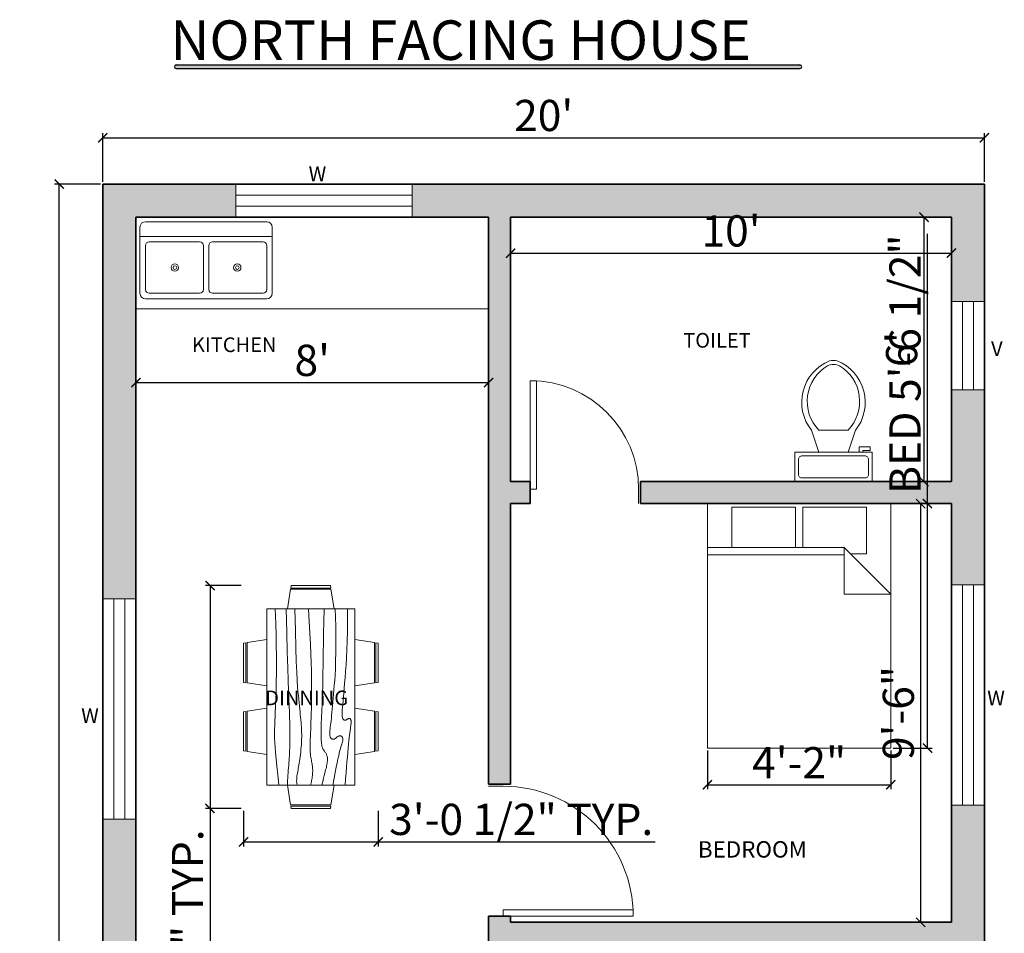
# Model space of a CAD drawing. Units: inches. Extents: x 3799 to 20199, y 1682 to 8087.
# Tile 29 of 30: x 17373 to 17641, y 7519 to 7768. Entities that reach past the tile are written whole.
import ezdxf

# ---------------------------------------------------------------- set-up
doc = ezdxf.new("R2010")
doc.units = ezdxf.units.IN
for name, color, linetype, lineweight in [('A-ANNO-DIMS', 2, 'Continuous', 18), ('A-ANNO-SYMB', 3, 'Continuous', 18), ('A-ANNO-TITL', 7, 'Continuous', 25), ('A-AREA-IDEN', 7, 'Continuous', 18), ('A-DOOR', 3, 'Continuous', 18), ('A-FLOR-CASE', 32, 'Continuous', 18), ('A-FLOR-FIXT', 9, 'Continuous', 18), ('A-FURN', 8, 'Continuous', 18), ('A-GLAZ', 152, 'Continuous', 18), ('A-WALL', 7, 'Continuous', 35), ('A-WALL-PATT', 252, 'Continuous', 13)]:
    doc.layers.add(name, color=color, linetype=linetype, lineweight=lineweight)
doc.styles.get("Standard").update_dxf_attribs({"font": 'arial.ttf'})
doc.dimstyles.new('ISO-25', dxfattribs={"dimtxt": 8.5, "dimasz": 2.5, "dimexe": 1.25, "dimexo": 0.625, "dimtad": 1, "dimdec": 0, "dimlunit": 3, "dimtxsty": 'Standard', "dimblk": 'ARCHTICK', "dimcen": 2.5, "dimadec": 0, "dimazin": 0, "dimtfac": 1, "dimtdec": 0, "dimtmove": 0, "dimatfit": 3, "dimfxl": 1, "dimarcsym": 0})

# ---------------------------------------------------------------- blocks, each defined once
blk = doc.blocks.new('*U47')
for p, q in [((0, 0), (0, -100)), ((750, 0), (750, -100))]:
    blk.add_line(p, q)
blk.add_lwpolyline([(0, 0), (0, 750), (43.75, 750), (43.75, 0)], close=True)
blk.add_arc((0, 0), 750, 0, 90)
blk = doc.blocks.new('*U124')
for p, q in [((0, 0), (0, -100)), ((-900, 0), (-900, -100))]:
    blk.add_line(p, q)
blk.add_lwpolyline([(0, 0), (0, 900), (-43.75, 900), (-43.75, 0)], close=True)
blk.add_arc((0, 0), 900, 90, 180)
blk = doc.blocks.new('Sink-double - 36 in top')
for p, q in [((-18, -4), (18, -4)), ((-0.75, -18.5), (-0.75, -6.5)), ((0.75, -6.5), (0.75, -18.5))]:
    blk.add_line(p, q)
for points in [[(-16.5, 0), (16.5, 0)], [(-18, -19.5), (-18, -1.5)], [(18, -1.5), (18, -19.5)], [(-16.5, -18.5), (-16.5, -6.5)], [(-15.5, -5.5), (-1.75, -5.5)], [(1.75, -5.5), (15.5, -5.5)], [(16.5, -6.5), (16.5, -18.5)], [(16.5, -21), (-16.5, -21)], [(-1.75, -19.5), (-15.5, -19.5)], [(15.5, -19.5), (1.75, -19.5)]]:
    blk.add_lwpolyline(points)
for centre, radius in [((-8.5, -12.5), 1), ((-8.5, -12.5), 0.5), ((8.5, -12.5), 1), ((8.5, -12.5), 0.5)]:
    blk.add_circle(centre, radius)
for centre, radius, start, end in [((-16.5, -1.5), 1.5, 90, 180), ((16.5, -1.5), 1.5, 0, 90), ((-15.5, -6.5), 1, 90, 180), ((-1.75, -6.5), 1, 0, 90), ((1.75, -6.5), 1, 90, 180), ((15.5, -6.5), 1, 0, 90), ((-15.5, -18.5), 1, 180, 270), ((-1.75, -18.5), 1, 270, 0), ((1.75, -18.5), 1, 180, 270), ((15.5, -18.5), 1, 270, 0), ((-16.5, -19.5), 1.5, 180, 270), ((16.5, -19.5), 1.5, 270, 0)]:
    blk.add_arc(centre, radius, start, end)
blk = doc.blocks.new('Toilet - top')
for p, q in [((9.5, -6), (9.5, -2)), ((-8, -8.5), (-8, -8)), ((-7, -8), (-7, -9.5)), ((-4, -8), (-6, -14)), ((4, -8), (6, -14)), ((-10, -8.5), (-8, -8.5)), ((-10, -9.5), (-10, -8.5)), ((-7, -9.5), (-10, -9.5)), ((4, -14), (-4, -14))]:
    blk.add_line(p, q)
blk.add_lwpolyline([(10.5, -8), (10.5, 0), (-10.5, 0), (-10.5, -8)], close=True)
for points in [[(-9.5, -2), (-9.5, -6)], [(8.5, -1), (-8.5, -1)], [(-8.5, -7), (8.5, -7)]]:
    blk.add_lwpolyline(points)
for centre, radius, start, end in [((-8.62, -1.88), 0.884, 81.8699, 188.1301), ((8.62, -1.88), 0.884, 351.8699, 98.1301), ((-8.62, -6.12), 0.884, 171.8699, 278.1301), ((8.62, -6.12), 0.884, 261.8699, 8.1301), ((3.52, -21.58), 12.17, 141.4691, 247.9714), ((4.2, -21.82), 11.33, 136.3677, 238.9468), ((-3.52, -21.58), 12.17, 292.0284, 38.5307), ((-4.2, -21.82), 11.33, 301.053, 43.6321), ((0, -27.88), 4, 245.7318, 294.2682), ((0, -29), 4, 254.8605, 285.1395)]:
    blk.add_arc(centre, radius, start, end)
blk = doc.blocks.new('Dining Set - 36 x 72 in.')
for p, q in [((-22.2343, 26.00059), (-23.4847, 17.99762)), ((-22.2304, 26), (-5.7608, 26)), ((-22, 27.5), (-22.1562, 26.50042)), ((-5.8416, 26.5), (-22.1534, 26.5)), ((-22, 27.5), (-6, 27.5)), ((-5.8437, 26.49966), (-6, 27.5)), ((-4.5152, 17.99762), (-5.7655, 25.99926)), ((5.7657, 26.00059), (4.5153, 17.99762)), ((5.7696, 26), (22.2392, 26)), ((6, 27.5), (5.8438, 26.50042)), ((22.1584, 26.5), (5.8466, 26.5)), ((6, 27.5), (22, 27.5)), ((22.1563, 26.49966), (22, 27.5)), ((23.4848, 17.99762), (22.2345, 25.99926)), ((36, 18), (-36, 18)), ((-36, 18), (-36, -18)), ((36, -18), (36, 18)), ((-45.5, 8), (-44.5004, 8.15617)), ((-44.5, -8.15843), (-44.5, 8.15338)), ((-44.0006, 8.23428), (-35.9976, 9.48474)), ((-44, 8.23041), (-44, -8.23915)), ((44.0006, 8.23428), (35.9976, 9.48474)), ((44, 8.23041), (44, -8.23915)), ((44.5, -8.15843), (44.5, 8.15338)), ((45.5, 8), (44.5005, 8.15617)), ((-45.5, 8), (-45.5, -8)), ((45.5, 8), (45.5, -8)), ((-44.4997, -8.15631), (-45.5, -8)), ((44.4997, -8.15631), (45.5, -8)), ((-35.9976, -9.48476), (-43.9993, -8.2345)), ((35.9976, -9.48476), (43.9993, -8.2345)), ((-36, -18), (36, -18)), ((-22.2343, -26.0006), (-23.4847, -17.99762)), ((-4.5152, -17.99762), (-5.7655, -25.99928)), ((5.7657, -26.0006), (4.5153, -17.99762)), ((23.4848, -17.99762), (22.2345, -25.99928)), ((-22.2304, -26), (-5.7608, -26)), ((-22, -27.5), (-22.1562, -26.50044)), ((-5.8416, -26.5), (-22.1534, -26.5)), ((-22, -27.5), (-6, -27.5)), ((-5.8437, -26.49967), (-6, -27.5)), ((5.7696, -26), (22.2392, -26)), ((6, -27.5), (5.8438, -26.50044)), ((22.1584, -26.5), (5.8466, -26.5)), ((6, -27.5), (22, -27.5)), ((22.1563, -26.49967), (22, -27.5))]:
    blk.add_line(p, q)
for points in [[(-36, 15), (-31.1772, 14.97754), (-26.8079, 14.91406), (-22.8538, 14.81543), (-19.276, 14.6875), (-16.0362, 14.53613), (-13.0957, 14.36718), (-10.4159, 14.18652), (-7.9583, 14), (-5.6904, 13.81315), (-3.6035, 13.63021), (-1.6954, 13.45508), (0.0365, 13.29166), (1.5945, 13.14388), (2.9811, 13.01562), (4.1988, 12.9108), (5.25, 12.83333), (6.1393, 12.78613), (6.8802, 12.76823), (7.4883, 12.77767), (7.9792, 12.8125), (8.3685, 12.87077), (8.6719, 12.95052), (8.9049, 13.0498), (9.0833, 13.16666), (9.2205, 13.29899), (9.3216, 13.44401), (9.3895, 13.59879), (9.4271, 13.76041), (9.4373, 13.92594), (9.4232, 14.09245), (9.3875, 14.257), (9.3333, 14.41666), (9.2638, 14.56917), (9.1836, 14.71484), (9.0975, 14.85465), (9.0104, 14.98958), (8.9272, 15.1206), (8.8529, 15.2487), (8.7922, 15.37483), (8.75, 15.5), (8.7305, 15.62467), (8.7344, 15.74739), (8.7617, 15.86621), (8.8125, 15.97916), (8.8867, 16.08431), (8.9844, 16.17968), (9.1055, 16.26334), (9.25, 16.33333), (9.4189, 16.38802), (9.6172, 16.42708), (9.8506, 16.45052), (10.125, 16.45833), (10.4463, 16.45052), (10.8203, 16.42708), (11.2529, 16.38802), (11.75, 16.33333), (12.3184, 16.26318), (12.9694, 16.17838), (13.7151, 16.07991), (14.5677, 15.96875), (15.5395, 15.84586), (16.6426, 15.71224), (17.8893, 15.56884), (19.2917, 15.41666), (20.859, 15.25667), (22.5879, 15.08984), (24.4721, 14.91715), (26.5052, 14.73958), (28.6809, 14.5581), (30.9929, 14.3737), (33.4347, 14.18733), (36, 14)], [(-36, 10), (-28.9766, 10.14274), (-23.1725, 10.20442), (-18.4241, 10.19775), (-14.5677, 10.13541), (-11.4399, 10.03011), (-8.877, 9.89453), (-6.7154, 9.74137), (-4.7917, 9.58333), (-2.9698, 9.43082), (-1.2246, 9.28515), (0.4415, 9.14534), (2.026, 9.01041), (3.5266, 8.87939), (4.9408, 8.7513), (6.266, 8.62516), (7.5, 8.5), (8.6411, 8.37549), (9.6914, 8.2539), (10.6538, 8.13818), (11.5312, 8.03125), (12.3267, 7.93603), (13.043, 7.85547), (13.6831, 7.79248), (14.25, 7.75), (14.7471, 7.7303), (15.1797, 7.73307), (15.5537, 7.75732), (15.875, 7.80208), (16.1494, 7.86637), (16.3828, 7.94922), (16.5811, 8.04964), (16.75, 8.16666), (16.8944, 8.29915), (17.0143, 8.44531), (17.1089, 8.60319), (17.1771, 8.77083), (17.218, 8.94629), (17.2305, 9.1276), (17.2137, 9.31282), (17.1667, 9.5), (17.0895, 9.6875), (16.987, 9.875), (16.8649, 10.0625), (16.7292, 10.25), (16.5856, 10.4375), (16.4401, 10.625), (16.2985, 10.8125), (16.1667, 11), (16.05, 11.18733), (15.9518, 11.3737), (15.8752, 11.5581), (15.8229, 11.73958), (15.798, 11.91715), (15.8034, 12.08984), (15.842, 12.25667), (15.9167, 12.41666), (16.0295, 12.56836), (16.1784, 12.70833), (16.3605, 12.83268), (16.5729, 12.9375), (16.8127, 13.01888), (17.0768, 13.07291), (17.3625, 13.0957), (17.6667, 13.08333), (17.9894, 13.03312), (18.3418, 12.94726), (18.7382, 12.82918), (19.1927, 12.68229), (19.7195, 12.51001), (20.3327, 12.31575), (21.0465, 12.10294), (21.875, 11.875), (22.8357, 11.63354), (23.959, 11.37304), (25.2786, 11.08618), (26.8282, 10.76562), (28.6414, 10.40405), (30.752, 9.99414), (33.1936, 9.52856), (36, 9)], [(-36, 5.5), (-30.7157, 5.3348), (-26.069, 5.20963), (-21.9946, 5.11767), (-18.4271, 5.05208), (-15.3009, 5.00602), (-12.5508, 4.97265), (-10.1112, 4.94515), (-7.9167, 4.91666), (-5.909, 4.88167), (-4.0586, 4.83984), (-2.3429, 4.79215), (-0.7396, 4.73958), (0.7739, 4.6831), (2.22, 4.6237), (3.6213, 4.56233), (5, 4.5), (6.373, 4.43782), (7.7344, 4.3776), (9.0723, 4.32129), (10.375, 4.27083), (11.6309, 4.22819), (12.8281, 4.19531), (13.9551, 4.17415), (15, 4.16666), (15.954, 4.17448), (16.819, 4.19791), (17.6001, 4.23698), (18.3021, 4.29166), (18.9299, 4.36198), (19.4883, 4.44791), (19.9823, 4.54948), (20.4167, 4.66666), (20.7969, 4.79899), (21.1302, 4.94401), (21.4245, 5.09879), (21.6875, 5.26041), (21.9271, 5.42594), (22.1511, 5.59245), (22.3672, 5.757), (22.5834, 5.91666), (22.8065, 6.06868), (23.0404, 6.21093), (23.2879, 6.34147), (23.5521, 6.45833), (23.8358, 6.55957), (24.142, 6.64323), (24.4735, 6.70735), (24.8334, 6.75), (25.2235, 6.76969), (25.642, 6.76692), (26.0858, 6.74267), (26.5521, 6.69791), (27.0379, 6.63362), (27.5404, 6.55078), (28.0565, 6.45036), (28.5834, 6.33333), (29.1242, 6.19987), (29.7071, 6.04687), (30.3661, 5.87044), (31.1354, 5.66666), (32.0493, 5.43164), (33.142, 5.16146), (34.4475, 4.85221), (36, 4.5)], [(-36, -1), (-30.7915, -0.6591), (-26.0195, -0.38216), (-21.6519, -0.16284), (-17.6563, 0.00521), (-14.0005, 0.12833), (-10.6523, 0.21289), (-7.5796, 0.26522), (-4.75, 0.29166), (-2.134, 0.29793), (0.2878, 0.28711), (2.5317, 0.26163), (4.6146, 0.22396), (6.5529, 0.17651), (8.3633, 0.12174), (10.0623, 0.06209), (11.6667, 0), (13.1899, -0.06201), (14.6341, -0.1211), (15.9982, -0.17432), (17.2813, -0.21875), (18.4823, -0.25147), (19.6003, -0.26953), (20.6343, -0.27002), (21.5834, -0.25), (22.4481, -0.20768), (23.2357, -0.14584), (23.9549, -0.06836), (24.6146, 0.02083), (25.2235, 0.11784), (25.7904, 0.21875), (26.3241, 0.31966), (26.8334, 0.41666), (27.3265, 0.50618), (27.8099, 0.58593), (28.2894, 0.65397), (28.7709, 0.70833), (29.2601, 0.74707), (29.763, 0.76823), (30.2855, 0.76985), (30.8334, 0.75), (31.4088, 0.70784), (31.9994, 0.64713), (32.589, 0.57275), (33.1615, 0.48958), (33.7008, 0.4025), (34.1908, 0.3164), (34.6153, 0.23616), (34.9584, 0.16666), (35.2099, 0.11165), (35.3848, 0.07031), (35.504, 0.04069), (35.5886, 0.02083), (35.6594, 0.00879), (35.7377, 0.0026), (35.8442, 0.00032), (36, 0)], [(-36, -6.5), (-27.1843, -6.31267), (-20.084, -6.1263), (-14.469, -5.9419), (-10.1094, -5.76042), (-6.7752, -5.58285), (-4.2363, -5.41016), (-2.2629, -5.24333), (-0.625, -5.08334), (0.8708, -4.93099), (2.2715, -4.78646), (3.5872, -4.64974), (4.8281, -4.52084), (6.0046, -4.39974), (7.127, -4.28646), (8.2053, -4.18099), (9.25, -4.08334), (10.2705, -3.99382), (11.2734, -3.91407), (12.2647, -3.84603), (13.25, -3.79167), (14.2354, -3.75293), (15.2266, -3.73177), (16.2295, -3.73015), (17.25, -3.75), (18.2912, -3.79248), (19.3451, -3.85547), (20.4009, -3.93604), (21.4479, -4.03125), (22.4754, -4.13819), (23.4727, -4.25391), (24.4289, -4.37549), (25.3334, -4.5), (26.1785, -4.62492), (26.9694, -4.74935), (27.7145, -4.87281), (28.4219, -4.99479), (29.1, -5.11483), (29.7572, -5.23242), (30.4016, -5.34709), (31.0417, -5.45834), (31.6837, -5.56437), (32.3262, -5.65821), (32.9658, -5.73153), (33.599, -5.77604), (34.2224, -5.78345), (34.8327, -5.74545), (35.4264, -5.65373), (36, -5.5)], [(-36, -10), (-26.4022, -9.81299), (-18.4675, -9.62891), (-11.9839, -9.45069), (-6.7396, -9.28125), (-2.5226, -9.12354), (0.8789, -8.98047), (3.6769, -8.85498), (6.0833, -8.75), (8.2767, -8.66765), (10.3021, -8.60677), (12.1712, -8.56543), (13.8958, -8.54167), (15.4876, -8.53353), (16.9583, -8.53907), (18.3197, -8.55632), (19.5834, -8.58334), (20.7616, -8.61841), (21.8685, -8.66081), (22.9188, -8.71004), (23.9271, -8.76563), (24.9081, -8.82707), (25.8763, -8.89388), (26.8465, -8.96558), (27.8334, -9.04167), (28.8474, -9.12118), (29.8828, -9.20117), (30.93, -9.27824), (31.9792, -9.34896), (33.0205, -9.40991), (34.0443, -9.45768), (35.0407, -9.48885), (36, -9.5)], [(-36, -14.5), (-30.0881, -14.33513), (-25.0332, -14.21224), (-20.7312, -14.12647), (-17.0781, -14.07292), (-13.97, -14.04671), (-11.3027, -14.04297), (-8.9724, -14.05681), (-6.875, -14.08334), (-4.9224, -14.11833), (-3.0905, -14.16016), (-1.3709, -14.20785), (0.2448, -14.26042), (1.7647, -14.3169), (3.1973, -14.3763), (4.5507, -14.43767), (5.8333, -14.5), (7.0554, -14.5621), (8.235, -14.62175), (9.3922, -14.67652), (10.5469, -14.72396), (11.7192, -14.76164), (12.929, -14.78711), (14.1965, -14.79794), (15.5417, -14.79167), (16.9933, -14.76424), (18.6152, -14.70508), (20.4804, -14.60197), (22.6615, -14.44271), (25.2312, -14.21509), (28.2624, -13.9069), (31.8277, -13.50594), (36, -13)]]:
    blk.add_lwpolyline(points)
blk = doc.blocks.new('Bed - Queen')
for p, q in [((0, -80.00003), (0, 0)), ((0, 0), (59.99999, 0)), ((59.99999, 0), (59.99999, -80.00003)), ((7.99999, -1.2), (28.79998, -1.2)), ((7.99999, -14.4), (7.99999, -1.2)), ((28.79998, -1.2), (28.79998, -14.4)), ((31.19999, -1.2), (51.99999, -1.2)), ((31.19999, -14.4), (31.19999, -1.2)), ((51.99999, -1.2), (51.99999, -16.4)), ((0, -14.4), (44.8, -14.4)), ((59.99999, -29.6), (44.8, -14.4)), ((44.8, -14.4), (44.8, -29.6)), ((44.8, -16.8), (0, -16.8)), ((51.99999, -16.4), (46.79936, -16.4)), ((44.8, -29.6), (59.99999, -29.6)), ((59.99999, -80.00003), (0, -80.00003))]:
    blk.add_line(p, q)
blk = doc.blocks.new('_ArchTick')
at = {"color": 0, "linetype": 'ByBlock', "const_width": 0.15}
blk.add_lwpolyline([(-0.5, -0.5), (0.5, 0.5)], dxfattribs=at)
blk = doc.blocks.new('*D159')
at = {"layer": 'A-ANNO-DIMS', "color": 0, "lineweight": -2, "transparency": 16777216}
for p, q in [((17404.17, 7688.47), (17404.17, 7667.72)), ((17500.17, 7688.47), (17500.17, 7667.72)), ((17404.17, 7668.97), (17500.17, 7668.97))]:
    blk.add_line(p, q, dxfattribs=at)
at = {"layer": 'Defpoints', "color": 0, "transparency": 16777216}
for p in [(17404.17, 7689.1), (17500.17, 7689.1), (17500.17, 7668.97)]:
    blk.add_point(p, dxfattribs=at)
at = {"layer": 'A-ANNO-DIMS', "color": 0, "lineweight": -2, "transparency": 16777216, "xscale": 2.5, "yscale": 2.5, "zscale": 2.5, "rotation": 180}
blk.add_blockref('_ArchTick', (17404.17, 7668.97), dxfattribs=at)
at = {"layer": 'A-ANNO-DIMS', "color": 0, "lineweight": -2, "transparency": 16777216, "xscale": 2.5, "yscale": 2.5, "zscale": 2.5}
blk.add_blockref('_ArchTick', (17500.17, 7668.97), dxfattribs=at)
at = {"layer": 'A-ANNO-DIMS', "color": 0, "transparency": 16777216, "insert": (17452.17, 7673.94), "char_height": 8.5, "attachment_point": 5}
blk.add_mtext("8'", dxfattribs=at)
blk = doc.blocks.new('*D160')
at = {"layer": 'A-ANNO-DIMS', "color": 0, "lineweight": -2, "transparency": 16777216}
for p, q in [((17506.17, 7713.39), (17506.17, 7702.98)), ((17626.17, 7713.39), (17626.17, 7702.98)), ((17506.17, 7704.23), (17626.17, 7704.23))]:
    blk.add_line(p, q, dxfattribs=at)
at = {"layer": 'Defpoints', "color": 0, "transparency": 16777216}
for p in [(17506.17, 7714.02), (17626.17, 7714.02), (17626.17, 7704.23)]:
    blk.add_point(p, dxfattribs=at)
at = {"layer": 'A-ANNO-DIMS', "color": 0, "lineweight": -2, "transparency": 16777216, "xscale": 2.5, "yscale": 2.5, "zscale": 2.5, "rotation": 180}
blk.add_blockref('_ArchTick', (17506.17, 7704.23), dxfattribs=at)
at = {"layer": 'A-ANNO-DIMS', "color": 0, "lineweight": -2, "transparency": 16777216, "xscale": 2.5, "yscale": 2.5, "zscale": 2.5}
blk.add_blockref('_ArchTick', (17626.17, 7704.23), dxfattribs=at)
at = {"layer": 'A-ANNO-DIMS', "color": 0, "transparency": 16777216, "insert": (17566.17, 7709.19), "char_height": 8.5, "attachment_point": 5}
blk.add_mtext("10'", dxfattribs=at)
blk = doc.blocks.new('*D161')
at = {"layer": 'A-ANNO-DIMS', "color": 0, "lineweight": -2, "transparency": 16777216}
for p, q in [((17625.55, 7714.02), (17617.44, 7714.02)), ((17618.69, 7714.02), (17618.69, 7642.02)), ((17625.55, 7642.02), (17617.44, 7642.02))]:
    blk.add_line(p, q, dxfattribs=at)
at = {"layer": 'Defpoints', "color": 0, "transparency": 16777216}
for p in [(17626.17, 7714.02), (17618.69, 7642.02), (17626.17, 7642.02)]:
    blk.add_point(p, dxfattribs=at)
at = {"layer": 'A-ANNO-DIMS', "color": 0, "lineweight": -2, "transparency": 16777216, "xscale": 2.5, "yscale": 2.5, "zscale": 2.5}
for p, rotation in [((17618.69, 7714.02), 90), ((17618.69, 7642.02), 270)]:
    blk.add_blockref('_ArchTick', p, dxfattribs=dict(at, rotation=rotation))
at = {"layer": 'A-ANNO-DIMS', "color": 0, "transparency": 16777216, "insert": (17613.72, 7678.02), "char_height": 8.5, "attachment_point": 5, "rotation": 90}
blk.add_mtext("6'", dxfattribs=at)
blk = doc.blocks.new('*D162')
at = {"layer": 'A-ANNO-DIMS', "color": 0, "lineweight": -2, "transparency": 16777216}
for p, q in [((17625.55, 7636.02), (17616.54, 7636.02)), ((17617.79, 7636.02), (17617.79, 7522.02)), ((17625.55, 7522.02), (17616.54, 7522.02))]:
    blk.add_line(p, q, dxfattribs=at)
at = {"layer": 'Defpoints', "color": 0, "transparency": 16777216}
for p in [(17626.17, 7636.02), (17617.79, 7522.02), (17626.17, 7522.02)]:
    blk.add_point(p, dxfattribs=at)
at = {"layer": 'A-ANNO-DIMS', "color": 0, "lineweight": -2, "transparency": 16777216, "xscale": 2.5, "yscale": 2.5, "zscale": 2.5}
for p, rotation in [((17617.79, 7636.02), 90), ((17617.79, 7522.02), 270)]:
    blk.add_blockref('_ArchTick', p, dxfattribs=dict(at, rotation=rotation))
at = {"layer": 'A-ANNO-DIMS', "color": 0, "transparency": 16777216, "insert": (17612.82, 7579.02), "char_height": 8.5, "attachment_point": 5, "rotation": 90}
blk.add_mtext('9\'-6"', dxfattribs=at)
blk = doc.blocks.new('*D168')
at = {"layer": 'A-ANNO-DIMS', "color": 0, "lineweight": -2, "transparency": 16777216}
for p, q in [((17395.17, 7723.64), (17395.17, 7736.91)), ((17395.17, 7735.66), (17635.17, 7735.66)), ((17635.17, 7723.64), (17635.17, 7736.91))]:
    blk.add_line(p, q, dxfattribs=at)
at = {"layer": 'Defpoints', "color": 0, "transparency": 16777216}
for p in [(17635.17, 7735.66), (17395.17, 7723.02), (17635.17, 7723.02)]:
    blk.add_point(p, dxfattribs=at)
at = {"layer": 'A-ANNO-DIMS', "color": 0, "lineweight": -2, "transparency": 16777216, "xscale": 2.5, "yscale": 2.5, "zscale": 2.5, "rotation": 180}
blk.add_blockref('_ArchTick', (17395.17, 7735.66), dxfattribs=at)
at = {"layer": 'A-ANNO-DIMS', "color": 0, "lineweight": -2, "transparency": 16777216, "xscale": 2.5, "yscale": 2.5, "zscale": 2.5}
blk.add_blockref('_ArchTick', (17635.17, 7735.66), dxfattribs=at)
at = {"layer": 'A-ANNO-DIMS', "color": 0, "transparency": 16777216, "insert": (17515.17, 7740.63), "char_height": 8.5, "attachment_point": 5}
blk.add_mtext("20'", dxfattribs=at)
blk = doc.blocks.new('*D169')
at = {"layer": 'A-ANNO-DIMS', "color": 0, "lineweight": -2, "transparency": 16777216}
for p, q in [((17394.55, 7723.02), (17382.05, 7723.02)), ((17383.3, 7243.02), (17383.3, 7723.02)), ((17394.55, 7243.02), (17382.05, 7243.02))]:
    blk.add_line(p, q, dxfattribs=at)
at = {"layer": 'Defpoints', "color": 0, "transparency": 16777216}
for p in [(17383.3, 7723.02), (17395.17, 7723.02), (17395.17, 7243.02)]:
    blk.add_point(p, dxfattribs=at)
at = {"layer": 'A-ANNO-DIMS', "color": 0, "lineweight": -2, "transparency": 16777216, "xscale": 2.5, "yscale": 2.5, "zscale": 2.5}
for p, rotation in [((17383.3, 7723.02), 90), ((17383.3, 7243.02), 270)]:
    blk.add_blockref('_ArchTick', p, dxfattribs=dict(at, rotation=rotation))
at = {"layer": 'A-ANNO-DIMS', "color": 0, "transparency": 16777216, "insert": (17378.33, 7483.02), "char_height": 8.5, "attachment_point": 5, "rotation": 90}
blk.add_mtext("40'", dxfattribs=at)
blk = doc.blocks.new('WIN-24IN-9IN-FRAME')
for p, q in [((0, 24), (9, 24)), ((3, 0), (3, 24)), ((6, 0), (6, 24)), ((0, 0), (9, 0))]:
    blk.add_line(p, q)
blk = doc.blocks.new('WIN-48IN-9IN-FRAME')
for p, q in [((0, 0), (0, 9)), ((48, 0), (48, 9)), ((48, 6), (0, 6)), ((48, 3), (0, 3))]:
    blk.add_line(p, q)
blk = doc.blocks.new('WIN-60IN-9IN-FRAME')
for p, q in [((0, 9), (0, 0)), ((60, 9), (60, 0)), ((60, 6), (0, 6)), ((60, 3), (0, 3))]:
    blk.add_line(p, q)
blk = doc.blocks.new('*D254')
at = {"layer": 'A-ANNO-DIMS', "color": 0, "lineweight": -2, "transparency": 16777216}
for p, q in [((17619.65, 7636.02), (17619.65, 7709.51)), ((17610.29, 7636.02), (17620.9, 7636.02)), ((17619.65, 7569.47), (17619.65, 7636.02)), ((17610.29, 7569.47), (17620.9, 7569.47))]:
    blk.add_line(p, q, dxfattribs=at)
at = {"layer": 'Defpoints', "color": 0, "transparency": 16777216}
for p in [(17609.67, 7636.02), (17619.65, 7636.02), (17609.67, 7569.47)]:
    blk.add_point(p, dxfattribs=at)
at = {"layer": 'A-ANNO-DIMS', "color": 0, "lineweight": -2, "transparency": 16777216, "xscale": 2.5, "yscale": 2.5, "zscale": 2.5}
for p, rotation in [((17619.65, 7636.02), 90), ((17619.65, 7569.47), 270)]:
    blk.add_blockref('_ArchTick', p, dxfattribs=dict(at, rotation=rotation))
at = {"layer": 'A-ANNO-DIMS', "color": 0, "transparency": 16777216, "insert": (17614.63, 7674.01), "char_height": 8.5, "attachment_point": 5, "rotation": 90}
blk.add_mtext('BED 5\'-6 1/2"', dxfattribs=at)
blk = doc.blocks.new('*D255')
at = {"layer": 'A-ANNO-DIMS', "color": 0, "lineweight": -2, "transparency": 16777216}
for p, q in [((17559.75, 7568.84), (17559.75, 7558.24)), ((17609.67, 7568.84), (17609.67, 7558.24)), ((17559.75, 7559.49), (17609.67, 7559.49))]:
    blk.add_line(p, q, dxfattribs=at)
at = {"layer": 'Defpoints', "color": 0, "transparency": 16777216}
for p in [(17559.75, 7569.47), (17609.67, 7569.47), (17609.67, 7559.49)]:
    blk.add_point(p, dxfattribs=at)
at = {"layer": 'A-ANNO-DIMS', "color": 0, "lineweight": -2, "transparency": 16777216, "xscale": 2.5, "yscale": 2.5, "zscale": 2.5, "rotation": 180}
blk.add_blockref('_ArchTick', (17559.75, 7559.49), dxfattribs=at)
at = {"layer": 'A-ANNO-DIMS', "color": 0, "lineweight": -2, "transparency": 16777216, "xscale": 2.5, "yscale": 2.5, "zscale": 2.5}
blk.add_blockref('_ArchTick', (17609.67, 7559.49), dxfattribs=at)
at = {"layer": 'A-ANNO-DIMS', "color": 0, "transparency": 16777216, "insert": (17584.71, 7564.38), "char_height": 8.5, "attachment_point": 5}
blk.add_mtext('4\'-2"', dxfattribs=at)
blk = doc.blocks.new('*D290')
at = {"layer": 'A-ANNO-DIMS', "color": 0, "lineweight": -2, "transparency": 16777216}
for p, q in [((17432.83, 7613.7), (17423.1, 7613.7)), ((17424.35, 7613.7), (17424.35, 7553.02)), ((17432.83, 7553.02), (17423.1, 7553.02)), ((17424.35, 7553.02), (17424.35, 7406.82))]:
    blk.add_line(p, q, dxfattribs=at)
at = {"layer": 'Defpoints', "color": 0, "transparency": 16777216}
for p in [(17433.46, 7613.7), (17424.35, 7553.02), (17433.46, 7553.02)]:
    blk.add_point(p, dxfattribs=at)
at = {"layer": 'A-ANNO-DIMS', "color": 0, "lineweight": -2, "transparency": 16777216, "xscale": 2.5, "yscale": 2.5, "zscale": 2.5}
for p, rotation in [((17424.35, 7613.7), 90), ((17424.35, 7553.02), 270)]:
    blk.add_blockref('_ArchTick', p, dxfattribs=dict(at, rotation=rotation))
at = {"layer": 'A-ANNO-DIMS', "color": 0, "transparency": 16777216, "insert": (17419.33, 7478.67), "char_height": 8.5, "attachment_point": 5, "rotation": 90}
blk.add_mtext('DINING SET 5\'-0 1/2" TYP.', dxfattribs=at)
blk = doc.blocks.new('*D291')
at = {"layer": 'A-ANNO-DIMS', "color": 0, "lineweight": -2, "transparency": 16777216}
for p, q in [((17433.46, 7552.4), (17433.46, 7542.67)), ((17470.13, 7552.4), (17470.13, 7542.67)), ((17433.46, 7543.92), (17470.13, 7543.92)), ((17470.13, 7543.92), (17545.49, 7543.92))]:
    blk.add_line(p, q, dxfattribs=at)
at = {"layer": 'Defpoints', "color": 0, "transparency": 16777216}
for p in [(17433.46, 7553.02), (17470.13, 7553.02), (17470.13, 7543.92)]:
    blk.add_point(p, dxfattribs=at)
at = {"layer": 'A-ANNO-DIMS', "color": 0, "lineweight": -2, "transparency": 16777216, "xscale": 2.5, "yscale": 2.5, "zscale": 2.5, "rotation": 180}
blk.add_blockref('_ArchTick', (17433.46, 7543.92), dxfattribs=at)
at = {"layer": 'A-ANNO-DIMS', "color": 0, "lineweight": -2, "transparency": 16777216, "xscale": 2.5, "yscale": 2.5, "zscale": 2.5}
blk.add_blockref('_ArchTick', (17470.13, 7543.92), dxfattribs=at)
at = {"layer": 'A-ANNO-DIMS', "color": 0, "transparency": 16777216, "insert": (17509.06, 7548.94), "char_height": 8.5, "attachment_point": 5}
blk.add_mtext('3\'-0 1/2" TYP.', dxfattribs=at)

msp = doc.modelspace()

# ---------------------------------------------------------------- hatches: boundary and pattern name
at = {"layer": 'A-ANNO-TITL'}
h = msp.add_hatch(color=256, dxfattribs=at)
h.dxf.hatch_style = 1
h.paths.add_polyline_path([(17584.94, 7755.5), (17415.14, 7755.5, 1), (17415.14, 7754.5), (17584.94, 7754.5, 1)])
at = {"layer": 'A-WALL-PATT'}
h = msp.add_hatch(color=256, dxfattribs=at)
h.dxf.hatch_style = 1
h.paths.add_polyline_path([(17635.17, 7553.93), (17626.17, 7553.93), (17626.17, 7522.02), (17506.17, 7522.02), (17506.17, 7523.65), (17500.17, 7523.65), (17500.17, 7516.02), (17626.17, 7516.02), (17626.17, 7505.71), (17635.17, 7505.71)])
h.paths.add_polyline_path([(17404.17, 7550.08), (17395.17, 7550.08), (17395.17, 7243.02), (17410.75, 7243.02), (17410.75, 7252.02), (17404.17, 7252.02)])
h.paths.add_polyline_path([(17635.17, 7469.71), (17626.17, 7469.71), (17626.17, 7456.02), (17554.17, 7456.02), (17554.17, 7450.02), (17626.17, 7450.02), (17626.17, 7405.75), (17635.17, 7405.75)])
h.paths.add_polyline_path([(17635.17, 7345.75), (17626.17, 7345.75), (17626.17, 7330.02), (17555.18, 7330.02, -0.022507), (17550.46, 7330.02), (17506.17, 7330.02), (17506.17, 7324.02), (17626.17, 7324.02), (17626.17, 7302.87), (17635.17, 7302.87)])
h.paths.add_polyline_path([(17635.17, 7266.87), (17626.17, 7266.87), (17626.17, 7252.02), (17569.79, 7252.02), (17569.79, 7243.02), (17635.17, 7243.02)])
h.paths.add_polyline_path([(17521.79, 7252.02), (17449.79, 7252.02, -0.03225), (17450.12, 7246.96), (17450.12, 7243.02), (17521.79, 7243.02)])
h.paths.add_polyline_path([(17431.36, 7723.02), (17395.17, 7723.02), (17395.17, 7610.08), (17404.17, 7610.08), (17404.17, 7714.02), (17431.36, 7714.02)])
h.paths.add_polyline_path([(17635.17, 7723.02), (17479.36, 7723.02), (17479.36, 7714.02), (17500.17, 7714.02), (17500.17, 7559.65), (17506.17, 7559.65), (17506.17, 7636.02), (17511.5, 7636.02), (17511.5, 7642.02), (17506.17, 7642.02), (17506.17, 7714.02), (17626.17, 7714.02), (17626.17, 7691.04), (17635.17, 7691.04)])
h.paths.add_polyline_path([(17635.17, 7667.04), (17626.17, 7667.04), (17626.17, 7642.02), (17541.5, 7642.02), (17541.5, 7636.02), (17626.17, 7636.02), (17626.17, 7613.93), (17635.17, 7613.93)], flags=17)

# ---------------------------------------------------------------- linework, layer by layer
at = {"layer": 'A-ANNO-TITL'}
for p, q in [((17415.14, 7755.5), (17584.94, 7755.5)), ((17415.14, 7754.5), (17584.94, 7754.5))]:
    msp.add_line(p, q, dxfattribs=at)
for centre, start, end in [((17415.14, 7755), 90, 270), ((17584.94, 7755), 270, 90)]:
    msp.add_arc(centre, 0.5, start, end, dxfattribs=at)
at = {"layer": 'A-FLOR-CASE'}
msp.add_line((17404.17, 7689.1), (17500.17, 7689.1), dxfattribs=at)
at = {"layer": 'A-WALL'}
for p, q in [((17395.17, 7723.02), (17635.17, 7723.02)), ((17395.17, 7243.02), (17395.17, 7723.02)), ((17635.17, 7723.02), (17635.17, 7243.02)), ((17404.17, 7714.02), (17500.17, 7714.02)), ((17404.17, 7252.02), (17404.17, 7714.02)), ((17500.17, 7714.02), (17500.17, 7559.65)), ((17506.17, 7714.02), (17506.17, 7642.02)), ((17506.17, 7714.02), (17626.17, 7714.02)), ((17626.17, 7714.02), (17626.17, 7642.02)), ((17506.17, 7642.02), (17511.5, 7642.02)), ((17511.5, 7636.02), (17511.5, 7642.02)), ((17541.5, 7636.02), (17541.5, 7642.02)), ((17541.5, 7642.02), (17626.17, 7642.02)), ((17506.17, 7636.02), (17511.5, 7636.02)), ((17506.17, 7636.02), (17506.17, 7559.65)), ((17541.5, 7636.02), (17626.17, 7636.02)), ((17626.17, 7636.02), (17626.17, 7522.02)), ((17506.17, 7559.65), (17500.17, 7559.65)), ((17506.17, 7523.65), (17500.17, 7523.65)), ((17500.17, 7523.65), (17500.17, 7516.02)), ((17506.17, 7523.65), (17506.17, 7522.02)), ((17506.17, 7522.02), (17626.17, 7522.02))]:
    msp.add_line(p, q, dxfattribs=at)

# ---------------------------------------------------------------- block references
at = {"layer": 'A-DOOR', "xscale": 0.0393700787401575, "yscale": 0.0393700787401575, "zscale": 0.0393700787401575}
msp.add_blockref('*U47', (17511.5, 7639.96), dxfattribs=at)
at = {"layer": 'A-DOOR', "xscale": 0.0393700787401575, "yscale": 0.0393700787401575, "zscale": 0.0393700787401575, "rotation": 270}
msp.add_blockref('*U124', (17504.11, 7523.65), dxfattribs=at)
at = {"layer": 'A-FLOR-FIXT'}
msp.add_blockref('Sink-double - 36 in top', (17423.28, 7712.81), dxfattribs=at)
at = {"layer": 'A-FLOR-FIXT', "rotation": 180}
msp.add_blockref('Toilet - top', (17594.06, 7642.02), dxfattribs=at)
at = {"layer": 'A-FURN', "xscale": 0.8318649475729376, "yscale": 0.8318649475729376, "zscale": 0.8318649475729376}
msp.add_blockref('Bed - Queen', (17559.75, 7636.02), dxfattribs=at)
at = {"layer": 'A-FURN', "xscale": 0.6667800638184667, "yscale": 0.6667800638184667, "zscale": 0.6667800638184667, "rotation": 270}
msp.add_blockref('Dining Set - 36 x 72 in.', (17451.79, 7583.36), dxfattribs=at)
at = {"layer": 'A-GLAZ'}
for name, p in [('WIN-48IN-9IN-FRAME', (17431.36, 7714.02)), ('WIN-24IN-9IN-FRAME', (17626.17, 7667.04))]:
    msp.add_blockref(name, p, dxfattribs=at)
at = {"layer": 'A-GLAZ', "rotation": 90}
for p in [(17635.17, 7553.93), (17404.17, 7550.08)]:
    msp.add_blockref('WIN-60IN-9IN-FRAME', p, dxfattribs=at)

# ---------------------------------------------------------------- texts
at = {"layer": 'A-ANNO-SYMB'}
for s, p in [('W', (17451.19, 7723.84)), ('V', (17636.97, 7676.2)), ('W', (17635.92, 7581.08)), ('W', (17389.28, 7576.3))]:
    msp.add_text(s, height=4, rotation=0.0011, dxfattribs=at).set_placement(p)
at = {"layer": 'A-ANNO-TITL'}
msp.add_text('NORTH FACING HOUSE', height=10.7706, rotation=0.0011, dxfattribs=at).set_placement((17413.57, 7756.85))
at = {"layer": 'A-AREA-IDEN'}
for s, height, p in [('TOILET', 4, (17553.16, 7678.5)), ('KITCHEN', 4, (17419.43, 7677.3)), ('DINNING', 4, (17439.38, 7581.13)), ('BEDROOM', 4.47, (17557.15, 7539.64))]:
    msp.add_text(s, height=height, rotation=0.0011, dxfattribs=at).set_placement(p)

# ---------------------------------------------------------------- dimensions: what is measured, and where the dimension line sits
at = {"layer": 'A-ANNO-DIMS'}
for base, p1, p2, override, picture, middle in [((17635.17, 7735.66), (17395.17, 7723.02), (17635.17, 7723.02), {"dimclrd": 0, "dimclre": 0, "dimclrt": 0}, '*D168', (17515.17, 7740.63)), ((17626.17, 7704.23), (17506.17, 7714.02), (17626.17, 7714.02), {"dimclrd": 0, "dimclre": 0, "dimclrt": 0}, '*D160', (17566.17, 7709.19)), ((17500.17, 7668.97), (17404.17, 7689.1), (17500.17, 7689.1), {"dimclrd": 0, "dimclre": 0, "dimclrt": 0}, '*D159', (17452.17, 7673.94)), ((17609.67, 7559.49), (17559.75, 7569.47), (17609.67, 7569.47), {"dimdec": 1, "dimlfac": 1, "dimrnd": 0, "dimzin": 1, "dimdsep": 46, "dimlunit": 4, "dimfrac": 2}, '*D255', (17584.71, 7564.38))]:
    dim = msp.add_linear_dim(base=base, p1=p1, p2=p2, dimstyle='ISO-25', override=override, dxfattribs=at)
    dim.commit()
    dim.dimension.update_dxf_attribs({"geometry": picture, "text_midpoint": middle})
for base, p1, p2, picture, middle in [((17383.3, 7723.02), (17395.17, 7243.02), (17395.17, 7723.02), '*D169', (17378.33, 7483.02)), ((17618.69, 7642.02), (17626.17, 7714.02), (17626.17, 7642.02), '*D161', (17613.72, 7678.02)), ((17617.79, 7522.02), (17626.17, 7636.02), (17626.17, 7522.02), '*D162', (17612.82, 7579.02))]:
    dim = msp.add_linear_dim(base=base, p1=p1, p2=p2, angle=90, dimstyle='ISO-25', override={"dimclrd": 0, "dimclre": 0, "dimclrt": 0}, dxfattribs=at)
    dim.commit()
    dim.dimension.update_dxf_attribs({"geometry": picture, "text_midpoint": middle})
for base, p1, p2, angle, text, picture, middle in [((17619.6477, 7636.0192), (17609.6653, 7569.47), (17609.6653, 7636.0192), 90, 'BED <>', '*D254', (17614.6278, 7674.0139)), ((17424.35, 7553.02), (17433.46, 7613.7), (17433.46, 7553.02), 270, 'DINING SET <> TYP.', '*D290', (17419.33, 7478.67))]:
    dim = msp.add_linear_dim(base=base, p1=p1, p2=p2, angle=angle, text=text, dimstyle='ISO-25', override={"dimdec": 1, "dimlfac": 1, "dimrnd": 0, "dimzin": 1, "dimdsep": 46, "dimlunit": 4, "dimfrac": 2}, dxfattribs=at)
    dim.commit()
    dim.dimension.update_dxf_attribs({"geometry": picture, "text_midpoint": middle})
dim = msp.add_linear_dim(base=(17470.13, 7543.92), p1=(17433.46, 7553.02), p2=(17470.13, 7553.02), text='<> TYP.', dimstyle='ISO-25', override={"dimdec": 1, "dimlfac": 1, "dimrnd": 0, "dimzin": 1, "dimdsep": 46, "dimlunit": 4, "dimfrac": 2}, dxfattribs=at)
dim.commit()
dim.dimension.update_dxf_attribs({"geometry": '*D291', "text_midpoint": (17509.06, 7548.94)})

doc.saveas('drawing.dxf')
